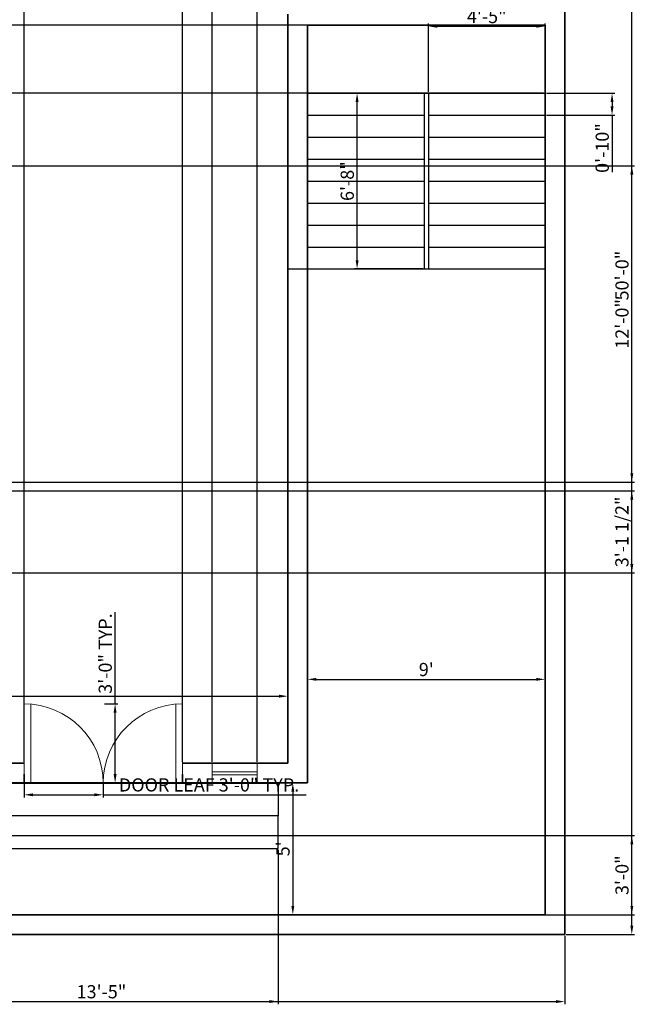
# Model space of a CAD drawing. Units: inches. Extents: x 1973 to 2661, y 1730 to 2412.
# Tile 4 of 5: x 2368 to 2652, y 1734 to 2182. Entities that reach past the tile are written whole.
import ezdxf

# ---------------------------------------------------------------- set-up
doc = ezdxf.new("R2010")
doc.units = ezdxf.units.IN
for name, color, linetype, lineweight in [('A-ANNO-DIMS', 2, 'Continuous', 18), ('A-DOOR', 3, 'Continuous', 18), ('A-FLOR-STRS', 7, 'Continuous', 25), ('A-GLAZ', 4, 'Continuous', 18), ('A-WALL', 7, 'Continuous', 35)]:
    doc.layers.add(name, color=color, linetype=linetype, lineweight=lineweight)
doc.styles.get("Standard").update_dxf_attribs({"font": 'arial.ttf'})
doc.dimstyles.new('ISO-25', dxfattribs={"dimtxt": 6, "dimasz": 4, "dimexe": 1.25, "dimexo": 0.625, "dimtad": 1, "dimdec": 0, "dimrnd": 6, "dimlunit": 3, "dimtxsty": 'Standard', "dimcen": 2.5, "dimadec": 0, "dimazin": 0, "dimtfac": 1, "dimtdec": 0, "dimtmove": 0, "dimatfit": 3, "dimfxl": 1, "dimarcsym": 0})

# ---------------------------------------------------------------- blocks, each defined once
blk = doc.blocks.new('*D4')
at = {"layer": 'A-ANNO-DIMS', "color": 0, "lineweight": -2, "transparency": 16777216}
for p, q in [((2499.04, 1834.98), (2499.04, 1882.77)), ((2503.04, 1881.52), (2603.04, 1881.52)), ((2607.04, 1834.98), (2607.04, 1882.77))]:
    blk.add_line(p, q, dxfattribs=at)
at = {"layer": 'A-ANNO-DIMS', "color": 0, "transparency": 16777216}
for points in [[(2503.04, 1882.18), (2503.04, 1880.85), (2499.04, 1881.52)], [(2603.04, 1882.18), (2603.04, 1880.85), (2607.04, 1881.52)]]:
    blk.add_solid(points, dxfattribs=at)
at = {"layer": 'Defpoints', "color": 0, "transparency": 16777216}
for p in [(2607.04, 1881.52), (2499.04, 1834.35), (2607.04, 1834.35)]:
    blk.add_point(p, dxfattribs=at)
at = {"layer": 'A-ANNO-DIMS', "color": 0, "transparency": 16777216, "insert": (2553.04, 1885.21), "char_height": 6, "attachment_point": 5}
blk.add_mtext("9'", dxfattribs=at)
blk = doc.blocks.new('*D5')
at = {"layer": 'A-ANNO-DIMS', "color": 0, "lineweight": -2, "transparency": 16777216}
for p, q in [((2498.42, 1834.35), (2491.06, 1834.35)), ((2492.31, 1830.35), (2492.31, 1778.35)), ((2498.42, 1774.35), (2491.06, 1774.35))]:
    blk.add_line(p, q, dxfattribs=at)
at = {"layer": 'A-ANNO-DIMS', "color": 0, "transparency": 16777216}
for points in [[(2491.64, 1830.35), (2492.98, 1830.35), (2492.31, 1834.35)], [(2491.64, 1778.35), (2492.98, 1778.35), (2492.31, 1774.35)]]:
    blk.add_solid(points, dxfattribs=at)
at = {"layer": 'Defpoints', "color": 0, "transparency": 16777216}
for p in [(2499.04, 1834.35), (2492.31, 1774.35), (2499.04, 1774.35)]:
    blk.add_point(p, dxfattribs=at)
at = {"layer": 'A-ANNO-DIMS', "color": 0, "transparency": 16777216, "insert": (2488.63, 1804.35), "char_height": 6, "attachment_point": 5, "rotation": 90}
blk.add_mtext("5'", dxfattribs=at)
blk = doc.blocks.new('DOOR-36-SWING')
for p, q in [((0, 0), (0, 36)), ((0, 36), (0, 0)), ((3, 0), (3, 36)), ((0, 0), (3, 0))]:
    blk.add_line(p, q)
blk.add_arc((0, 0), 36, 0, 90)
blk = doc.blocks.new('*D18')
at = {"layer": 'A-ANNO-DIMS', "color": 0, "lineweight": -2, "transparency": 16777216}
for p, q in [((2370.04, 1833.73), (2370.04, 1827.7)), ((2406.04, 1833.73), (2406.04, 1827.7)), ((2374.04, 1828.95), (2402.04, 1828.95)), ((2406.04, 1828.95), (2498.33, 1828.95))]:
    blk.add_line(p, q, dxfattribs=at)
at = {"layer": 'A-ANNO-DIMS', "color": 0, "transparency": 16777216}
for points in [[(2374.04, 1829.62), (2374.04, 1828.28), (2370.04, 1828.95)], [(2402.04, 1829.62), (2402.04, 1828.28), (2406.04, 1828.95)]]:
    blk.add_solid(points, dxfattribs=at)
at = {"layer": 'Defpoints', "color": 0, "transparency": 16777216}
for p in [(2370.04, 1834.35), (2406.04, 1834.35), (2406.04, 1828.95)]:
    blk.add_point(p, dxfattribs=at)
at = {"layer": 'A-ANNO-DIMS', "color": 0, "transparency": 16777216, "insert": (2454.19, 1832.68), "char_height": 6, "attachment_point": 5}
blk.add_mtext('DOOR LEAF 3\'-0" TYP.', dxfattribs=at)
blk = doc.blocks.new('*D19')
at = {"layer": 'A-ANNO-DIMS', "color": 0, "lineweight": -2, "transparency": 16777216}
for p, q in [((2411.44, 1870.35), (2411.44, 1912.17)), ((2406.67, 1870.35), (2412.69, 1870.35)), ((2411.44, 1838.35), (2411.44, 1866.35)), ((2406.67, 1834.35), (2412.69, 1834.35))]:
    blk.add_line(p, q, dxfattribs=at)
at = {"layer": 'A-ANNO-DIMS', "color": 0, "transparency": 16777216}
for points in [[(2410.78, 1866.35), (2412.11, 1866.35), (2411.44, 1870.35)], [(2410.78, 1838.35), (2412.11, 1838.35), (2411.44, 1834.35)]]:
    blk.add_solid(points, dxfattribs=at)
at = {"layer": 'Defpoints', "color": 0, "transparency": 16777216}
for p in [(2406.04, 1870.35), (2411.44, 1870.35), (2406.04, 1834.35)]:
    blk.add_point(p, dxfattribs=at)
at = {"layer": 'A-ANNO-DIMS', "color": 0, "transparency": 16777216, "insert": (2407.75, 1893.26), "char_height": 6, "attachment_point": 5, "rotation": 90}
blk.add_mtext('3\'-0" TYP.', dxfattribs=at)
blk = doc.blocks.new('*D30')
at = {"layer": 'A-ANNO-DIMS', "color": 0, "lineweight": -2, "transparency": 16777216}
for p, q in [((2016.04, 1764.73), (2016.04, 1733.57)), ((2616.04, 1764.73), (2616.04, 1733.57)), ((2020.04, 1734.82), (2612.04, 1734.82))]:
    blk.add_line(p, q, dxfattribs=at)
at = {"layer": 'A-ANNO-DIMS', "color": 0, "transparency": 16777216}
for points in [[(2020.04, 1735.49), (2020.04, 1734.15), (2016.04, 1734.82)], [(2612.04, 1735.49), (2612.04, 1734.15), (2616.04, 1734.82)]]:
    blk.add_solid(points, dxfattribs=at)
at = {"layer": 'Defpoints', "color": 0, "transparency": 16777216}
for p in [(2016.04, 1765.35), (2616.04, 1765.35), (2616.04, 1734.82)]:
    blk.add_point(p, dxfattribs=at)
at = {"layer": 'A-ANNO-DIMS', "color": 0, "transparency": 16777216, "insert": (2316.04, 1738.51), "char_height": 6, "attachment_point": 5}
blk.add_mtext('50\'-0"', dxfattribs=at)
blk = doc.blocks.new('*D31')
at = {"layer": 'A-ANNO-DIMS', "color": 0, "lineweight": -2, "transparency": 16777216}
for p, q in [((2616.67, 2365.35), (2647.79, 2365.35)), ((2646.54, 1769.35), (2646.54, 2361.35)), ((2616.67, 1765.35), (2647.79, 1765.35))]:
    blk.add_line(p, q, dxfattribs=at)
at = {"layer": 'A-ANNO-DIMS', "color": 0, "transparency": 16777216}
for points in [[(2645.88, 2361.35), (2647.21, 2361.35), (2646.54, 2365.35)], [(2645.88, 1769.35), (2647.21, 1769.35), (2646.54, 1765.35)]]:
    blk.add_solid(points, dxfattribs=at)
at = {"layer": 'Defpoints', "color": 0, "transparency": 16777216}
for p in [(2616.04, 2365.35), (2646.54, 2365.35), (2616.04, 1765.35)]:
    blk.add_point(p, dxfattribs=at)
at = {"layer": 'A-ANNO-DIMS', "color": 0, "transparency": 16777216, "insert": (2642.85, 2065.35), "char_height": 6, "attachment_point": 5, "rotation": 90}
blk.add_mtext('50\'-0"', dxfattribs=at)
blk = doc.blocks.new('*D53')
at = {"layer": 'A-ANNO-DIMS', "color": 0, "lineweight": -2, "transparency": 16777216}
for p, q in [((2197.04, 1843.98), (2197.04, 1875.1)), ((2201.04, 1873.85), (2486.04, 1873.85)), ((2490.04, 1843.98), (2490.04, 1875.1))]:
    blk.add_line(p, q, dxfattribs=at)
at = {"layer": 'A-ANNO-DIMS', "color": 0, "transparency": 16777216}
for points in [[(2201.04, 1874.52), (2201.04, 1873.18), (2197.04, 1873.85)], [(2486.04, 1874.52), (2486.04, 1873.18), (2490.04, 1873.85)]]:
    blk.add_solid(points, dxfattribs=at)
at = {"layer": 'Defpoints', "color": 0, "transparency": 16777216}
for p in [(2490.04, 1873.85), (2197.04, 1843.35), (2490.04, 1843.35)]:
    blk.add_point(p, dxfattribs=at)
at = {"layer": 'A-ANNO-DIMS', "color": 0, "transparency": 16777216, "insert": (2343.54, 1877.54), "char_height": 6, "attachment_point": 5}
blk.add_mtext('24\'-5"', dxfattribs=at)
blk = doc.blocks.new('*D57')
at = {"layer": 'A-ANNO-DIMS', "color": 0, "lineweight": -2, "transparency": 16777216}
for p, q in [((2193.67, 1810.35), (2647.79, 1810.35)), ((2646.54, 1778.35), (2646.54, 1806.35)), ((2193.67, 1774.35), (2647.79, 1774.35))]:
    blk.add_line(p, q, dxfattribs=at)
at = {"layer": 'A-ANNO-DIMS', "color": 0, "transparency": 16777216}
for points in [[(2645.88, 1806.35), (2647.21, 1806.35), (2646.54, 1810.35)], [(2645.88, 1778.35), (2647.21, 1778.35), (2646.54, 1774.35)]]:
    blk.add_solid(points, dxfattribs=at)
at = {"layer": 'Defpoints', "color": 0, "transparency": 16777216}
for p in [(2193.04, 1810.35), (2646.54, 1810.35), (2193.04, 1774.35)]:
    blk.add_point(p, dxfattribs=at)
at = {"layer": 'A-ANNO-DIMS', "color": 0, "transparency": 16777216, "insert": (2642.85, 1792.35), "char_height": 6, "attachment_point": 5, "rotation": 90}
blk.add_mtext('3\'-0"', dxfattribs=at)
blk = doc.blocks.new('*D59')
at = {"layer": 'A-ANNO-DIMS', "color": 0, "lineweight": -2, "transparency": 16777216}
for p, q in [((2193.67, 2115.35), (2647.79, 2115.35)), ((2646.54, 1975.35), (2646.54, 2111.35)), ((2193.67, 1971.35), (2647.79, 1971.35))]:
    blk.add_line(p, q, dxfattribs=at)
at = {"layer": 'A-ANNO-DIMS', "color": 0, "transparency": 16777216}
for points in [[(2645.88, 2111.35), (2647.21, 2111.35), (2646.54, 2115.35)], [(2645.88, 1975.35), (2647.21, 1975.35), (2646.54, 1971.35)]]:
    blk.add_solid(points, dxfattribs=at)
at = {"layer": 'Defpoints', "color": 0, "transparency": 16777216}
for p in [(2193.04, 2115.35), (2646.54, 2115.35), (2193.04, 1971.35)]:
    blk.add_point(p, dxfattribs=at)
at = {"layer": 'A-ANNO-DIMS', "color": 0, "transparency": 16777216, "insert": (2642.85, 2043.35), "char_height": 6, "attachment_point": 5, "rotation": 90}
blk.add_mtext('12\'-0"', dxfattribs=at)
blk = doc.blocks.new('*D60')
at = {"layer": 'A-ANNO-DIMS', "color": 0, "lineweight": -2, "transparency": 16777216}
for p, q in [((2551.42, 2148.35), (2520.29, 2148.35)), ((2521.54, 2072.35), (2521.54, 2144.35)), ((2551.42, 2068.35), (2520.29, 2068.35))]:
    blk.add_line(p, q, dxfattribs=at)
at = {"layer": 'A-ANNO-DIMS', "color": 0, "transparency": 16777216}
for points in [[(2520.88, 2144.35), (2522.21, 2144.35), (2521.54, 2148.35)], [(2520.88, 2072.35), (2522.21, 2072.35), (2521.54, 2068.35)]]:
    blk.add_solid(points, dxfattribs=at)
at = {"layer": 'Defpoints', "color": 0, "transparency": 16777216}
for p in [(2521.54, 2148.35), (2552.04, 2148.35), (2552.04, 2068.35)]:
    blk.add_point(p, dxfattribs=at)
at = {"layer": 'A-ANNO-DIMS', "color": 0, "transparency": 16777216, "insert": (2517.85, 2108.35), "char_height": 6, "attachment_point": 5, "rotation": 90}
blk.add_mtext('6\'-8"', dxfattribs=at)
blk = doc.blocks.new('*D61')
at = {"layer": 'A-ANNO-DIMS', "color": 0, "lineweight": -2, "transparency": 16777216}
for p, q in [((2606.42, 2179.35), (1984.22, 2179.35)), ((1985.47, 2152.35), (1985.47, 2175.35)), ((2606.42, 2148.35), (1984.22, 2148.35))]:
    blk.add_line(p, q, dxfattribs=at)
at = {"layer": 'A-ANNO-DIMS', "color": 0, "transparency": 16777216}
for points in [[(1984.81, 2175.35), (1986.14, 2175.35), (1985.47, 2179.35)], [(1984.81, 2152.35), (1986.14, 2152.35), (1985.47, 2148.35)]]:
    blk.add_solid(points, dxfattribs=at)
at = {"layer": 'Defpoints', "color": 0, "transparency": 16777216}
for p in [(1985.47, 2179.35), (2607.04, 2179.35), (2607.04, 2148.35)]:
    blk.add_point(p, dxfattribs=at)
at = {"layer": 'A-ANNO-DIMS', "color": 0, "transparency": 16777216, "insert": (1981.84, 2163.85), "char_height": 6, "attachment_point": 5, "rotation": 90}
blk.add_mtext('2\'-7"', dxfattribs=at)
blk = doc.blocks.new('*D62')
at = {"layer": 'A-ANNO-DIMS', "color": 0, "lineweight": -2, "transparency": 16777216}
for p, q in [((2607.67, 2148.35), (2638.79, 2148.35)), ((2637.54, 2144.35), (2637.54, 2142.35)), ((2607.67, 2138.35), (2638.79, 2138.35)), ((2637.54, 2138.35), (2637.54, 2112.49))]:
    blk.add_line(p, q, dxfattribs=at)
at = {"layer": 'A-ANNO-DIMS', "color": 0, "transparency": 16777216}
for points in [[(2636.88, 2144.35), (2638.21, 2144.35), (2637.54, 2148.35)], [(2636.88, 2142.35), (2638.21, 2142.35), (2637.54, 2138.35)]]:
    blk.add_solid(points, dxfattribs=at)
at = {"layer": 'Defpoints', "color": 0, "transparency": 16777216}
for p in [(2607.04, 2148.35), (2607.04, 2138.35), (2637.54, 2138.35)]:
    blk.add_point(p, dxfattribs=at)
at = {"layer": 'A-ANNO-DIMS', "color": 0, "transparency": 16777216, "insert": (2633.85, 2123.42), "char_height": 6, "attachment_point": 5, "rotation": 90}
blk.add_mtext('0\'-10"', dxfattribs=at)
blk = doc.blocks.new('*D63')
at = {"layer": 'A-ANNO-DIMS', "color": 0, "lineweight": -2, "transparency": 16777216}
for p, q in [((2554.04, 2148.98), (2554.04, 2180.1)), ((2558.04, 2178.85), (2603.04, 2178.85)), ((2607.04, 2148.98), (2607.04, 2180.1))]:
    blk.add_line(p, q, dxfattribs=at)
at = {"layer": 'A-ANNO-DIMS', "color": 0, "transparency": 16777216}
for points in [[(2558.04, 2179.52), (2558.04, 2178.18), (2554.04, 2178.85)], [(2603.04, 2179.52), (2603.04, 2178.18), (2607.04, 2178.85)]]:
    blk.add_solid(points, dxfattribs=at)
at = {"layer": 'Defpoints', "color": 0, "transparency": 16777216}
for p in [(2607.04, 2178.85), (2554.04, 2148.35), (2607.04, 2148.35)]:
    blk.add_point(p, dxfattribs=at)
at = {"layer": 'A-ANNO-DIMS', "color": 0, "transparency": 16777216, "insert": (2580.54, 2182.53), "char_height": 6, "attachment_point": 5}
blk.add_mtext('4\'-5"', dxfattribs=at)
blk = doc.blocks.new('*D65')
at = {"layer": 'A-ANNO-DIMS', "color": 0, "lineweight": -2, "transparency": 16777216}
for p, q in [((2324.79, 1803.83), (2324.79, 1733.57)), ((2485.69, 1803.83), (2485.69, 1733.57)), ((2328.79, 1734.82), (2481.69, 1734.82))]:
    blk.add_line(p, q, dxfattribs=at)
at = {"layer": 'A-ANNO-DIMS', "color": 0, "transparency": 16777216}
for points in [[(2328.79, 1735.49), (2328.79, 1734.15), (2324.79, 1734.82)], [(2481.69, 1735.49), (2481.69, 1734.15), (2485.69, 1734.82)]]:
    blk.add_solid(points, dxfattribs=at)
at = {"layer": 'Defpoints', "color": 0, "transparency": 16777216}
for p in [(2324.79, 1804.45), (2485.69, 1804.45), (2485.69, 1734.82)]:
    blk.add_point(p, dxfattribs=at)
at = {"layer": 'A-ANNO-DIMS', "color": 0, "transparency": 16777216, "insert": (2405.24, 1738.51), "char_height": 6, "attachment_point": 5}
blk.add_mtext('13\'-5"', dxfattribs=at)
blk = doc.blocks.new('*D67')
at = {"layer": 'A-ANNO-DIMS', "color": 0, "lineweight": -2, "transparency": 16777216}
for p, q in [((2455.64, 1843.98), (2455.64, 2397.1)), ((2459.64, 2395.85), (2472.06, 2395.85)), ((2476.06, 1843.98), (2476.06, 2397.1)), ((2476.06, 2395.85), (2510.68, 2395.85))]:
    blk.add_line(p, q, dxfattribs=at)
at = {"layer": 'A-ANNO-DIMS', "color": 0, "transparency": 16777216}
for points in [[(2459.64, 2396.52), (2459.64, 2395.18), (2455.64, 2395.85)], [(2472.06, 2396.52), (2472.06, 2395.18), (2476.06, 2395.85)]]:
    blk.add_solid(points, dxfattribs=at)
at = {"layer": 'Defpoints', "color": 0, "transparency": 16777216}
for p in [(2476.06, 2395.85), (2455.64, 1843.35), (2476.06, 1843.35)]:
    blk.add_point(p, dxfattribs=at)
at = {"layer": 'A-ANNO-DIMS', "color": 0, "transparency": 16777216, "insert": (2495.37, 2399.58), "char_height": 6, "attachment_point": 5}
blk.add_mtext('1\'-8 1/2"', dxfattribs=at)
blk = doc.blocks.new('*D68')
at = {"layer": 'A-ANNO-DIMS', "color": 0, "lineweight": -2, "transparency": 16777216}
for p, q in [((2442.04, 1843.98), (2442.04, 2397.1)), ((2446.04, 2395.85), (2451.64, 2395.85)), ((2455.64, 1843.98), (2455.64, 2397.1)), ((2455.64, 2395.85), (2490.26, 2395.85))]:
    blk.add_line(p, q, dxfattribs=at)
at = {"layer": 'A-ANNO-DIMS', "color": 0, "transparency": 16777216}
for points in [[(2446.04, 2396.52), (2446.04, 2395.18), (2442.04, 2395.85)], [(2451.64, 2396.52), (2451.64, 2395.18), (2455.64, 2395.85)]]:
    blk.add_solid(points, dxfattribs=at)
at = {"layer": 'Defpoints', "color": 0, "transparency": 16777216}
for p in [(2455.64, 2395.85), (2442.04, 1843.35), (2455.64, 1843.35)]:
    blk.add_point(p, dxfattribs=at)
at = {"layer": 'A-ANNO-DIMS', "color": 0, "transparency": 16777216, "insert": (2474.95, 2399.58), "char_height": 6, "attachment_point": 5}
blk.add_mtext('1\'-1 1/2"', dxfattribs=at)
blk = doc.blocks.new('*D69')
at = {"layer": 'A-ANNO-DIMS', "color": 0, "lineweight": -2, "transparency": 16777216}
for p, q in [((2357.02, 1843.98), (2357.02, 2397.1)), ((2361.02, 2395.85), (2366.04, 2395.85)), ((2370.04, 1843.98), (2370.04, 2397.1)), ((2370.04, 2395.85), (2390.68, 2395.85))]:
    blk.add_line(p, q, dxfattribs=at)
at = {"layer": 'A-ANNO-DIMS', "color": 0, "transparency": 16777216}
for points in [[(2361.02, 2396.52), (2361.02, 2395.18), (2357.02, 2395.85)], [(2366.04, 2396.52), (2366.04, 2395.18), (2370.04, 2395.85)]]:
    blk.add_solid(points, dxfattribs=at)
at = {"layer": 'Defpoints', "color": 0, "transparency": 16777216}
for p in [(2370.04, 2395.85), (2357.02, 1843.35), (2370.04, 1843.35)]:
    blk.add_point(p, dxfattribs=at)
at = {"layer": 'A-ANNO-DIMS', "color": 0, "transparency": 16777216, "insert": (2382.36, 2399.49), "char_height": 6, "attachment_point": 5}
blk.add_mtext('1\'-1"', dxfattribs=at)
blk = doc.blocks.new('*D73')
at = {"layer": 'A-ANNO-DIMS', "color": 0, "lineweight": -2, "transparency": 16777216}
for p, q in [((2066.89, 1967.35), (2647.79, 1967.35)), ((2646.54, 1933.97), (2646.54, 1963.35)), ((2066.89, 1929.97), (2647.79, 1929.97))]:
    blk.add_line(p, q, dxfattribs=at)
at = {"layer": 'A-ANNO-DIMS', "color": 0, "transparency": 16777216}
for points in [[(2645.88, 1963.35), (2647.21, 1963.35), (2646.54, 1967.35)], [(2645.88, 1933.97), (2647.21, 1933.97), (2646.54, 1929.97)]]:
    blk.add_solid(points, dxfattribs=at)
at = {"layer": 'Defpoints', "color": 0, "transparency": 16777216}
for p in [(2066.26, 1967.35), (2646.54, 1967.35), (2066.26, 1929.97)]:
    blk.add_point(p, dxfattribs=at)
at = {"layer": 'A-ANNO-DIMS', "color": 0, "transparency": 16777216, "insert": (2642.81, 1948.66), "char_height": 6, "attachment_point": 5, "rotation": 90}
blk.add_mtext('3\'-1 1/2"', dxfattribs=at)

msp = doc.modelspace()

# ---------------------------------------------------------------- linework, layer by layer
at = {"layer": 'A-FLOR-STRS'}
for p, q in [((2499.04, 2148.35), (2607.04, 2148.35)), ((2552.04, 2148.35), (2552.04, 2068.35)), ((2554.04, 2148.35), (2554.04, 2068.35)), ((2499.04, 2138.35), (2552.04, 2138.35)), ((2554.04, 2138.35), (2607.04, 2138.35)), ((2499.04, 2128.35), (2552.04, 2128.35)), ((2554.04, 2128.35), (2607.04, 2128.35)), ((2499.04, 2118.35), (2552.04, 2118.35)), ((2554.04, 2118.35), (2607.04, 2118.35)), ((2499.04, 2108.35), (2552.04, 2108.35)), ((2554.04, 2108.35), (2607.04, 2108.35)), ((2499.04, 2098.35), (2552.04, 2098.35)), ((2554.04, 2098.35), (2607.04, 2098.35)), ((2499.04, 2088.35), (2552.04, 2088.35)), ((2554.04, 2088.35), (2607.04, 2088.35)), ((2499.04, 2078.35), (2552.04, 2078.35)), ((2554.04, 2078.35), (2607.04, 2078.35)), ((2490.04, 2068.35), (2607.04, 2068.35)), ((2324.79, 1834.25), (2485.69, 1834.25)), ((2485.69, 1834.25), (2485.69, 1819.35)), ((2485.69, 1819.35), (2324.79, 1819.35)), ((2485.69, 1819.35), (2324.79, 1819.35)), ((2485.69, 1804.45), (2485.69, 1819.35)), ((2324.79, 1804.45), (2485.69, 1804.45))]:
    msp.add_line(p, q, dxfattribs=at)
at = {"layer": 'A-GLAZ'}
for p, q in [((2476.06, 1843.35), (2455.64, 1843.35)), ((2455.64, 1843.35), (2455.64, 1834.35)), ((2476.06, 1834.35), (2476.06, 1843.35)), ((2476.06, 1839.42), (2455.64, 1839.42)), ((2455.64, 1834.35), (2455.64, 1838.06)), ((2455.64, 1838.06), (2476.06, 1838.06)), ((2476.06, 1838.06), (2476.06, 1839.42))]:
    msp.add_line(p, q, dxfattribs=at)
at = {"layer": 'A-WALL'}
for p, q in [((2616.04, 2365.35), (2616.04, 1765.35)), ((2490.04, 2184.35), (2490.04, 1843.35)), ((2607.04, 2179.35), (2499.04, 2179.35)), ((2499.04, 2179.35), (2499.04, 1834.35)), ((2607.04, 1774.35), (2607.04, 2179.35)), ((2370.04, 1843.35), (2197.04, 1843.35)), ((2490.04, 1843.35), (2442.04, 1843.35)), ((2370.04, 1838.35), (2370.04, 1834.35)), ((2442.04, 1838.35), (2442.04, 1834.35)), ((2197.04, 1834.35), (2499.04, 1834.35)), ((2499.04, 1834.35), (2476.06, 1834.35)), ((2197.04, 1774.35), (2607.04, 1774.35)), ((2616.04, 1765.35), (2016.04, 1765.35))]:
    msp.add_line(p, q, dxfattribs=at)

# ---------------------------------------------------------------- block references
at = {"layer": 'A-DOOR'}
msp.add_blockref('DOOR-36-SWING', (2370.04, 1834.35), dxfattribs=at)
at = {"layer": 'A-DOOR', "extrusion": (0, 0, -1), "zscale": -1}
msp.add_blockref('DOOR-36-SWING', (-2442.04, 1834.35), dxfattribs=at)

# ---------------------------------------------------------------- dimensions: what is measured, and where the dimension line sits
at = {"layer": 'A-ANNO-DIMS'}
for base, p1, p2, override, picture, middle in [((2455.64, 2395.85), (2442.04, 1843.35), (2455.64, 1843.35), {"dimdec": 1, "dimlfac": 1, "dimrnd": 0, "dimzin": 1, "dimdsep": 46, "dimlunit": 4, "dimfrac": 2}, '*D68', (2474.95, 2399.58)), ((2476.06, 2395.85), (2455.64, 1843.35), (2476.06, 1843.35), {"dimdec": 1, "dimlfac": 1, "dimrnd": 0, "dimzin": 1, "dimdsep": 46, "dimlunit": 4, "dimfrac": 2}, '*D67', (2495.37, 2399.58)), ((2370.04, 2395.85), (2357.02, 1843.35), (2370.04, 1843.35), {"dimdec": 1, "dimlfac": 1, "dimrnd": 0, "dimzin": 1, "dimdsep": 46, "dimlunit": 4, "dimfrac": 2}, '*D69', (2382.36, 2399.49)), ((2607.04, 2178.85), (2554.04, 2148.35), (2607.04, 2148.35), {"dimdec": 1, "dimlfac": 1, "dimrnd": 0, "dimzin": 1, "dimdsep": 46, "dimlunit": 4, "dimfrac": 2}, '*D63', (2580.54, 2182.53)), ((2607.04, 1881.52), (2499.04, 1834.35), (2607.04, 1834.35), {"dimclrd": 0, "dimclre": 0, "dimclrt": 0}, '*D4', (2553.04, 1885.21)), ((2490.04, 1873.85), (2197.04, 1843.35), (2490.04, 1843.35), {"dimdec": 1, "dimlfac": 1, "dimrnd": 0, "dimzin": 1, "dimdsep": 46, "dimlunit": 4, "dimfrac": 2}, '*D53', (2343.54, 1877.54)), ((2485.69, 1734.82), (2324.79, 1804.45), (2485.69, 1804.45), {"dimdec": 1, "dimlfac": 1, "dimrnd": 0, "dimzin": 1, "dimdsep": 46, "dimlunit": 4, "dimfrac": 2}, '*D65', (2405.24, 1738.51)), ((2616.04, 1734.82), (2016.04, 1765.35), (2616.04, 1765.35), {"dimdec": 1, "dimlfac": 1, "dimrnd": 0, "dimzin": 1, "dimdsep": 46, "dimlunit": 4, "dimfrac": 2}, '*D30', (2316.04, 1738.51))]:
    dim = msp.add_linear_dim(base=base, p1=p1, p2=p2, dimstyle='ISO-25', override=override, dxfattribs=at)
    dim.commit()
    dim.dimension.update_dxf_attribs({"geometry": picture, "text_midpoint": middle})
for base, p1, p2, angle, override, picture, middle in [((2646.54, 2365.35), (2616.04, 1765.35), (2616.04, 2365.35), 90, {"dimdec": 1, "dimlfac": 1, "dimrnd": 0, "dimzin": 1, "dimdsep": 46, "dimlunit": 4, "dimfrac": 2}, '*D31', (2642.85, 2065.35)), ((1985.47, 2179.35), (2607.04, 2148.35), (2607.04, 2179.35), 90, {"dimdec": 1, "dimlfac": 1, "dimrnd": 0, "dimzin": 1, "dimdsep": 46, "dimlunit": 4, "dimfrac": 2}, '*D61', (1981.84, 2163.85)), ((2521.54, 2148.35), (2552.04, 2068.35), (2552.04, 2148.35), 90, {"dimdec": 1, "dimlfac": 1, "dimrnd": 0, "dimzin": 1, "dimdsep": 46, "dimlunit": 4, "dimfrac": 2}, '*D60', (2517.85, 2108.35)), ((2637.54, 2138.35), (2607.04, 2148.35), (2607.04, 2138.35), 270, {"dimdec": 1, "dimlfac": 1, "dimrnd": 0, "dimzin": 1, "dimdsep": 46, "dimlunit": 4, "dimfrac": 2}, '*D62', (2633.85, 2123.42)), ((2646.54, 2115.35), (2193.04, 1971.35), (2193.04, 2115.35), 90, {"dimdec": 1, "dimlfac": 1, "dimrnd": 0, "dimzin": 1, "dimdsep": 46, "dimlunit": 4, "dimfrac": 2}, '*D59', (2642.85, 2043.35)), ((2646.54, 1967.35), (2066.26, 1929.97), (2066.26, 1967.35), 90, {"dimdec": 1, "dimlfac": 1, "dimrnd": 0, "dimzin": 1, "dimdsep": 46, "dimlunit": 4, "dimfrac": 2}, '*D73', (2642.81, 1948.66)), ((2492.31, 1774.35), (2499.04, 1834.35), (2499.04, 1774.35), 90, {"dimclrd": 0, "dimclre": 0, "dimclrt": 0}, '*D5', (2488.63, 1804.35)), ((2646.54, 1810.35), (2193.04, 1774.35), (2193.04, 1810.35), 90, {"dimdec": 1, "dimlfac": 1, "dimrnd": 0, "dimzin": 1, "dimdsep": 46, "dimlunit": 4, "dimfrac": 2}, '*D57', (2642.85, 1792.35))]:
    dim = msp.add_linear_dim(base=base, p1=p1, p2=p2, angle=angle, dimstyle='ISO-25', override=override, dxfattribs=at)
    dim.commit()
    dim.dimension.update_dxf_attribs({"geometry": picture, "text_midpoint": middle})
dim = msp.add_linear_dim(base=(2411.44, 1870.35), p1=(2406.04, 1834.35), p2=(2406.04, 1870.35), angle=90, text='<> TYP.', dimstyle='ISO-25', override={"dimdec": 1, "dimlfac": 1, "dimrnd": 0, "dimzin": 1, "dimdsep": 46, "dimlunit": 4, "dimfrac": 2}, dxfattribs=at)
dim.commit()
dim.dimension.update_dxf_attribs({"geometry": '*D19', "text_midpoint": (2407.75, 1893.26)})
dim = msp.add_linear_dim(base=(2406.04, 1828.95), p1=(2370.04, 1834.35), p2=(2406.04, 1834.35), text='DOOR LEAF <> TYP.', dimstyle='ISO-25', override={"dimdec": 1, "dimlfac": 1, "dimrnd": 0, "dimzin": 1, "dimdsep": 46, "dimlunit": 4, "dimfrac": 2}, dxfattribs=at)
dim.commit()
dim.dimension.update_dxf_attribs({"geometry": '*D18', "text_midpoint": (2454.19, 1832.68)})

doc.saveas('drawing.dxf')
